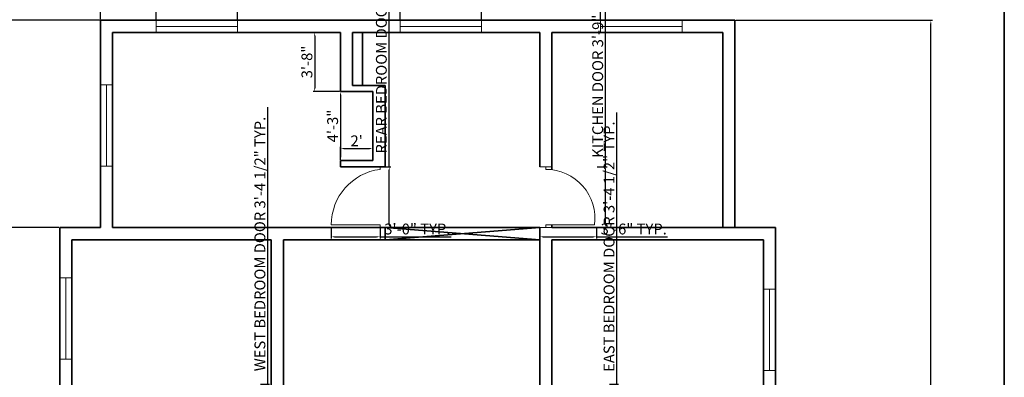
# Model space of a CAD drawing. Units: inches. Extents: x 2257 to 3678, y 834 to 1975.
# Tile 8 of 16: x 2952 to 3678, y 1330 to 1594. Entities that reach past the tile are written whole.
import ezdxf

# ---------------------------------------------------------------- set-up
doc = ezdxf.new("R2010")
doc.units = ezdxf.units.IN
for name, color, linetype, lineweight in [('A-ANNO-DIMS', 2, 'Continuous', 18), ('A-ANNO-TTLB', 7, 'Continuous', 35), ('A-DOOR', 3, 'Continuous', 18), ('A-GLAZ', 4, 'Continuous', 18), ('A-WALL', 7, 'Continuous', 35)]:
    doc.layers.add(name, color=color, linetype=linetype, lineweight=lineweight)
doc.styles.get("Standard").update_dxf_attribs({"font": 'arial.ttf'})
doc.dimstyles.new('ISO-25', dxfattribs={"dimtxt": 8, "dimasz": 2.5, "dimexe": 1.25, "dimexo": 0.625, "dimtad": 1, "dimdec": 0, "dimlunit": 3, "dimtxsty": 'Standard', "dimcen": 2.5, "dimadec": 0, "dimazin": 0, "dimtfac": 1, "dimtdec": 0, "dimtmove": 0, "dimatfit": 3, "dimfxl": 1, "dimarcsym": 0})

# ---------------------------------------------------------------- blocks, each defined once
blk = doc.blocks.new('*D17')
at = {"layer": 'A-ANNO-DIMS', "color": 0, "lineweight": -2, "transparency": 16777216}
for p, q in [((3187.62, 1584.58), (3168.03, 1584.58)), ((3169.28, 1582.08), (3169.28, 1543.58)), ((3187.62, 1541.08), (3168.03, 1541.08))]:
    blk.add_line(p, q, dxfattribs=at)
at = {"layer": 'A-ANNO-DIMS', "color": 0, "transparency": 16777216}
for points in [[(3168.87, 1582.08), (3169.7, 1582.08), (3169.28, 1584.58)], [(3168.87, 1543.58), (3169.7, 1543.58), (3169.28, 1541.08)]]:
    blk.add_solid(points, dxfattribs=at)
at = {"layer": 'Defpoints', "color": 0, "transparency": 16777216}
for p in [(3188.24, 1584.58), (3169.28, 1541.08), (3188.24, 1541.08)]:
    blk.add_point(p, dxfattribs=at)
at = {"layer": 'A-ANNO-DIMS', "color": 0, "transparency": 16777216, "insert": (3164.57, 1562.83), "char_height": 8, "attachment_point": 5, "rotation": 90}
blk.add_mtext('3\'-8"', dxfattribs=at)
blk = doc.blocks.new('*D18')
at = {"layer": 'A-ANNO-DIMS', "color": 0, "lineweight": -2, "transparency": 16777216}
for p, q in [((3188.87, 1541.08), (3189.49, 1541.08)), ((3188.24, 1538.58), (3188.24, 1492.58)), ((3188.87, 1490.08), (3189.49, 1490.08))]:
    blk.add_line(p, q, dxfattribs=at)
at = {"layer": 'A-ANNO-DIMS', "color": 0, "transparency": 16777216}
for points in [[(3187.82, 1538.58), (3188.66, 1538.58), (3188.24, 1541.08)], [(3187.82, 1492.58), (3188.66, 1492.58), (3188.24, 1490.08)]]:
    blk.add_solid(points, dxfattribs=at)
at = {"layer": 'Defpoints', "color": 0, "transparency": 16777216}
for p in [(3188.24, 1541.08), (3188.24, 1490.08), (3188.24, 1490.08)]:
    blk.add_point(p, dxfattribs=at)
at = {"layer": 'A-ANNO-DIMS', "color": 0, "transparency": 16777216, "insert": (3183.53, 1515.58), "char_height": 8, "attachment_point": 5, "rotation": 90}
blk.add_mtext('4\'-3"', dxfattribs=at)
blk = doc.blocks.new('*D15')
at = {"layer": 'A-ANNO-DIMS', "color": 0, "lineweight": -2, "transparency": 16777216}
for p, q in [((3188.24, 1490.7), (3188.24, 1500.22)), ((3190.74, 1498.97), (3209.74, 1498.97)), ((3212.24, 1490.7), (3212.24, 1500.22))]:
    blk.add_line(p, q, dxfattribs=at)
at = {"layer": 'A-ANNO-DIMS', "color": 0, "transparency": 16777216}
for points in [[(3190.74, 1499.38), (3190.74, 1498.55), (3188.24, 1498.97)], [(3209.74, 1499.38), (3209.74, 1498.55), (3212.24, 1498.97)]]:
    blk.add_solid(points, dxfattribs=at)
at = {"layer": 'Defpoints', "color": 0, "transparency": 16777216}
for p in [(3212.24, 1498.97), (3188.24, 1490.08), (3212.24, 1490.08)]:
    blk.add_point(p, dxfattribs=at)
at = {"layer": 'A-ANNO-DIMS', "color": 0, "transparency": 16777216, "insert": (3200.24, 1503.61), "char_height": 8, "attachment_point": 5}
blk.add_mtext("2'", dxfattribs=at)
blk = doc.blocks.new('WIN-60')
for p, q in [((0, 9), (0, 0)), ((60, 4.5), (60, 9)), ((60, 9), (60, 0)), ((0, 0), (0, 4.5)), ((0, 4.5), (60, 4.5))]:
    blk.add_line(p, q)
blk = doc.blocks.new('WIN-60-SIDE')
for p, q in [((0, 60), (9, 60)), ((9, 60), (4.5, 60)), ((4.5, 60), (4.5, 0)), ((9, 0), (0, 0)), ((4.5, 0), (9, 0))]:
    blk.add_line(p, q)
blk = doc.blocks.new('DOOR-BEDROOM-REAR')
for p, q in [((36, 45), (36, 43)), ((36, 2), (0, 2)), ((36, 0), (36, 2))]:
    blk.add_line(p, q)
blk.add_arc((41.35, 2), 41.35, 97.43058, 180)
blk = doc.blocks.new('DOOR-KITCHEN')
for p, q in [((0, 45), (9, 45)), ((4.5, 45), (4.5, 43)), ((9, 45), (4.5, 45)), ((4.5, 0), (4.5, 2)), ((4.5, 2), (40.5, 2)), ((9, 0), (0, 0))]:
    blk.add_line(p, q)
blk.add_arc((4.5, 6.7), 36.3, 352.56942, 90)
blk = doc.blocks.new('*D62')
at = {"layer": 'A-ANNO-DIMS', "color": 0, "lineweight": -2, "transparency": 16777216}
for p, q in [((3224.23, 1485.58), (3224.23, 1669.32)), ((3218.11, 1485.58), (3225.48, 1485.58)), ((3224.23, 1443.08), (3224.23, 1483.08)), ((3218.11, 1440.58), (3225.48, 1440.58))]:
    blk.add_line(p, q, dxfattribs=at)
at = {"layer": 'A-ANNO-DIMS', "color": 0, "transparency": 16777216}
for points in [[(3223.82, 1483.08), (3224.65, 1483.08), (3224.23, 1485.58)], [(3223.82, 1443.08), (3224.65, 1443.08), (3224.23, 1440.58)]]:
    blk.add_solid(points, dxfattribs=at)
at = {"layer": 'Defpoints', "color": 0, "transparency": 16777216}
for p in [(3217.48, 1485.58), (3224.23, 1485.58), (3217.48, 1440.58)]:
    blk.add_point(p, dxfattribs=at)
at = {"layer": 'A-ANNO-DIMS', "color": 0, "transparency": 16777216, "insert": (3219.47, 1578.7), "char_height": 8, "attachment_point": 5, "rotation": 90}
blk.add_mtext('REAR BEDROOM DOOR 3\'-9" TYP.', dxfattribs=at)
blk = doc.blocks.new('*D63')
at = {"layer": 'A-ANNO-DIMS', "color": 0, "lineweight": -2, "transparency": 16777216}
for p, q in [((3181.48, 1439.95), (3181.48, 1432.58)), ((3217.48, 1439.95), (3217.48, 1432.58)), ((3183.98, 1433.83), (3214.98, 1433.83)), ((3217.48, 1433.83), (3269.99, 1433.83))]:
    blk.add_line(p, q, dxfattribs=at)
at = {"layer": 'A-ANNO-DIMS', "color": 0, "transparency": 16777216}
for points in [[(3183.98, 1434.24), (3183.98, 1433.41), (3181.48, 1433.83)], [(3214.98, 1434.24), (3214.98, 1433.41), (3217.48, 1433.83)]]:
    blk.add_solid(points, dxfattribs=at)
at = {"layer": 'Defpoints', "color": 0, "transparency": 16777216}
for p in [(3181.48, 1440.58), (3217.48, 1440.58), (3217.48, 1433.83)]:
    blk.add_point(p, dxfattribs=at)
at = {"layer": 'A-ANNO-DIMS', "color": 0, "transparency": 16777216, "insert": (3244.99, 1438.54), "char_height": 8, "attachment_point": 5}
blk.add_mtext('3\'-0" TYP.', dxfattribs=at)
blk = doc.blocks.new('*D64')
at = {"layer": 'A-ANNO-DIMS', "color": 0, "lineweight": -2, "transparency": 16777216}
for p, q in [((3134.67, 1325.08), (3134.67, 1529.43)), ((3129.22, 1325.08), (3135.92, 1325.08)), ((3134.67, 1287.08), (3134.67, 1322.58)), ((3129.22, 1284.58), (3135.92, 1284.58))]:
    blk.add_line(p, q, dxfattribs=at)
at = {"layer": 'A-ANNO-DIMS', "color": 0, "transparency": 16777216}
for points in [[(3134.25, 1322.58), (3135.09, 1322.58), (3134.67, 1325.08)], [(3134.25, 1287.08), (3135.09, 1287.08), (3134.67, 1284.58)]]:
    blk.add_solid(points, dxfattribs=at)
at = {"layer": 'Defpoints', "color": 0, "transparency": 16777216}
for p in [(3128.6, 1325.08), (3134.67, 1325.08), (3128.6, 1284.58)]:
    blk.add_point(p, dxfattribs=at)
at = {"layer": 'A-ANNO-DIMS', "color": 0, "transparency": 16777216, "insert": (3129.9, 1428.5), "char_height": 8, "attachment_point": 5, "rotation": 90}
blk.add_mtext('WEST BEDROOM DOOR 3\'-4 1/2" TYP.', dxfattribs=at)
blk = doc.blocks.new('*D66')
at = {"layer": 'A-ANNO-DIMS', "color": 0, "lineweight": -2, "transparency": 16777216}
for p, q in [((3392.2, 1325.08), (3392.2, 1525.59)), ((3386.75, 1325.08), (3393.45, 1325.08)), ((3392.2, 1287.08), (3392.2, 1322.58)), ((3386.75, 1284.58), (3393.45, 1284.58))]:
    blk.add_line(p, q, dxfattribs=at)
at = {"layer": 'A-ANNO-DIMS', "color": 0, "transparency": 16777216}
for points in [[(3391.79, 1322.58), (3392.62, 1322.58), (3392.2, 1325.08)], [(3391.79, 1287.08), (3392.62, 1287.08), (3392.2, 1284.58)]]:
    blk.add_solid(points, dxfattribs=at)
at = {"layer": 'Defpoints', "color": 0, "transparency": 16777216}
for p in [(3386.13, 1325.08), (3392.2, 1325.08), (3386.13, 1284.58)]:
    blk.add_point(p, dxfattribs=at)
at = {"layer": 'A-ANNO-DIMS', "color": 0, "transparency": 16777216, "insert": (3387.44, 1426.58), "char_height": 8, "attachment_point": 5, "rotation": 90}
blk.add_mtext('EAST BEDROOM DOOR 3\'-4 1/2" TYP.', dxfattribs=at)
blk = doc.blocks.new('*D70')
at = {"layer": 'A-ANNO-DIMS', "color": 0, "lineweight": -2, "transparency": 16777216}
for p, q in [((3383.84, 1485.58), (3383.84, 1626.53)), ((3377.72, 1485.58), (3385.09, 1485.58)), ((3383.84, 1443.08), (3383.84, 1483.08)), ((3377.72, 1440.58), (3385.09, 1440.58))]:
    blk.add_line(p, q, dxfattribs=at)
at = {"layer": 'A-ANNO-DIMS', "color": 0, "transparency": 16777216}
for points in [[(3383.42, 1483.08), (3384.26, 1483.08), (3383.84, 1485.58)], [(3383.42, 1443.08), (3384.26, 1443.08), (3383.84, 1440.58)]]:
    blk.add_solid(points, dxfattribs=at)
at = {"layer": 'Defpoints', "color": 0, "transparency": 16777216}
for p in [(3377.09, 1485.58), (3383.84, 1485.58), (3377.09, 1440.58)]:
    blk.add_point(p, dxfattribs=at)
at = {"layer": 'A-ANNO-DIMS', "color": 0, "transparency": 16777216, "insert": (3379.07, 1557.3), "char_height": 8, "attachment_point": 5, "rotation": 90}
blk.add_mtext('KITCHEN DOOR 3\'-9" TYP.', dxfattribs=at)
blk = doc.blocks.new('*D71')
at = {"layer": 'A-ANNO-DIMS', "color": 0, "lineweight": -2, "transparency": 16777216}
for p, q in [((3335.24, 1439.95), (3335.24, 1432.58)), ((3377.09, 1439.95), (3377.09, 1432.58)), ((3337.74, 1433.83), (3374.59, 1433.83)), ((3377.09, 1433.83), (3429.6, 1433.83))]:
    blk.add_line(p, q, dxfattribs=at)
at = {"layer": 'A-ANNO-DIMS', "color": 0, "transparency": 16777216}
for points in [[(3337.74, 1434.24), (3337.74, 1433.41), (3335.24, 1433.83)], [(3374.59, 1434.24), (3374.59, 1433.41), (3377.09, 1433.83)]]:
    blk.add_solid(points, dxfattribs=at)
at = {"layer": 'Defpoints', "color": 0, "transparency": 16777216}
for p in [(3335.24, 1440.58), (3377.09, 1440.58), (3377.09, 1433.83)]:
    blk.add_point(p, dxfattribs=at)
at = {"layer": 'A-ANNO-DIMS', "color": 0, "transparency": 16777216, "insert": (3404.6, 1438.54), "char_height": 8, "attachment_point": 5}
blk.add_mtext('3\'-6" TYP.', dxfattribs=at)
blk = doc.blocks.new('*D100')
at = {"layer": 'A-ANNO-DIMS', "color": 0, "lineweight": -2, "transparency": 16777216}
for p, q in [((3479.87, 1593.58), (3625.01, 1593.58)), ((3623.76, 931.6), (3623.76, 1591.08)), ((3369.06, 929.1), (3625.01, 929.1))]:
    blk.add_line(p, q, dxfattribs=at)
at = {"layer": 'A-ANNO-DIMS', "color": 0, "transparency": 16777216}
for points in [[(3623.34, 1591.08), (3624.17, 1591.08), (3623.76, 1593.58)], [(3623.34, 931.6), (3624.17, 931.6), (3623.76, 929.1)]]:
    blk.add_solid(points, dxfattribs=at)
at = {"layer": 'Defpoints', "color": 0, "transparency": 16777216}
for p in [(3479.24, 1593.58), (3623.76, 1593.58), (3368.44, 929.1)]:
    blk.add_point(p, dxfattribs=at)
at = {"layer": 'A-ANNO-DIMS', "color": 0, "transparency": 16777216, "insert": (3618.99, 1261.34), "char_height": 8, "attachment_point": 5, "rotation": 90}
blk.add_mtext('55\'-4 1/2"', dxfattribs=at)
blk = doc.blocks.new('*D103')
at = {"layer": 'A-ANNO-DIMS', "color": 0, "lineweight": -2, "transparency": 16777216}
for p, q in [((2980.62, 1440.58), (2896.72, 1440.58)), ((2897.97, 1287.08), (2897.97, 1438.08)), ((2980.62, 1284.58), (2896.72, 1284.58))]:
    blk.add_line(p, q, dxfattribs=at)
at = {"layer": 'A-ANNO-DIMS', "color": 0, "transparency": 16777216}
for points in [[(2897.55, 1438.08), (2898.38, 1438.08), (2897.97, 1440.58)], [(2897.55, 1287.08), (2898.38, 1287.08), (2897.97, 1284.58)]]:
    blk.add_solid(points, dxfattribs=at)
at = {"layer": 'Defpoints', "color": 0, "transparency": 16777216}
for p in [(2897.97, 1440.58), (2981.24, 1440.58), (2981.24, 1284.58)]:
    blk.add_point(p, dxfattribs=at)
at = {"layer": 'A-ANNO-DIMS', "color": 0, "transparency": 16777216, "insert": (2893.25, 1362.58), "char_height": 8, "attachment_point": 5, "rotation": 90}
blk.add_mtext('13\'-0"', dxfattribs=at)
blk = doc.blocks.new('*D104')
at = {"layer": 'A-ANNO-DIMS', "color": 0, "lineweight": -2, "transparency": 16777216}
for p, q in [((3010.62, 1593.58), (2896.72, 1593.58)), ((2897.97, 1443.08), (2897.97, 1591.08)), ((2980.62, 1440.58), (2896.72, 1440.58))]:
    blk.add_line(p, q, dxfattribs=at)
at = {"layer": 'A-ANNO-DIMS', "color": 0, "transparency": 16777216}
for points in [[(2897.55, 1591.08), (2898.38, 1591.08), (2897.97, 1593.58)], [(2897.55, 1443.08), (2898.38, 1443.08), (2897.97, 1440.58)]]:
    blk.add_solid(points, dxfattribs=at)
at = {"layer": 'Defpoints', "color": 0, "transparency": 16777216}
for p in [(2897.97, 1593.58), (3011.24, 1593.58), (2981.24, 1440.58)]:
    blk.add_point(p, dxfattribs=at)
at = {"layer": 'A-ANNO-DIMS', "color": 0, "transparency": 16777216, "insert": (2893.26, 1517.08), "char_height": 8, "attachment_point": 5, "rotation": 90}
blk.add_mtext('12\'-9"', dxfattribs=at)
blk = doc.blocks.new('*D108')
at = {"layer": 'A-ANNO-DIMS', "color": 0, "lineweight": -2, "transparency": 16777216}
for p, q in [((3011.24, 1594.2), (3011.24, 1628.38)), ((3013.74, 1627.13), (3049.79, 1627.13)), ((3052.29, 1594.2), (3052.29, 1628.38))]:
    blk.add_line(p, q, dxfattribs=at)
at = {"layer": 'A-ANNO-DIMS', "color": 0, "transparency": 16777216}
for points in [[(3013.74, 1627.54), (3013.74, 1626.71), (3011.24, 1627.13)], [(3049.79, 1627.54), (3049.79, 1626.71), (3052.29, 1627.13)]]:
    blk.add_solid(points, dxfattribs=at)
at = {"layer": 'Defpoints', "color": 0, "transparency": 16777216}
for p in [(3052.29, 1627.13), (3011.24, 1593.58), (3052.29, 1593.58)]:
    blk.add_point(p, dxfattribs=at)
at = {"layer": 'A-ANNO-DIMS', "color": 0, "transparency": 16777216, "insert": (3031.77, 1631.84), "char_height": 8, "attachment_point": 5}
blk.add_mtext('3\'-5"', dxfattribs=at)
blk = doc.blocks.new('*D109')
at = {"layer": 'A-ANNO-DIMS', "color": 0, "lineweight": -2, "transparency": 16777216}
for p, q in [((3112.29, 1594.2), (3112.29, 1628.38)), ((3114.79, 1627.13), (3229.89, 1627.13)), ((3232.39, 1594.2), (3232.39, 1628.38))]:
    blk.add_line(p, q, dxfattribs=at)
at = {"layer": 'A-ANNO-DIMS', "color": 0, "transparency": 16777216}
for points in [[(3114.79, 1627.54), (3114.79, 1626.71), (3112.29, 1627.13)], [(3229.89, 1627.54), (3229.89, 1626.71), (3232.39, 1627.13)]]:
    blk.add_solid(points, dxfattribs=at)
at = {"layer": 'Defpoints', "color": 0, "transparency": 16777216}
for p in [(3232.39, 1627.13), (3112.29, 1593.58), (3232.39, 1593.58)]:
    blk.add_point(p, dxfattribs=at)
at = {"layer": 'A-ANNO-DIMS', "color": 0, "transparency": 16777216, "insert": (3172.34, 1631.84), "char_height": 8, "attachment_point": 5}
blk.add_mtext('10\'-0"', dxfattribs=at)
blk = doc.blocks.new('*D110')
at = {"layer": 'A-ANNO-DIMS', "color": 0, "lineweight": -2, "transparency": 16777216}
for p, q in [((3292.39, 1594.2), (3292.39, 1628.38)), ((3294.89, 1627.13), (3377.71, 1627.13)), ((3380.21, 1594.2), (3380.21, 1628.38))]:
    blk.add_line(p, q, dxfattribs=at)
at = {"layer": 'A-ANNO-DIMS', "color": 0, "transparency": 16777216}
for points in [[(3294.89, 1627.54), (3294.89, 1626.71), (3292.39, 1627.13)], [(3377.71, 1627.54), (3377.71, 1626.71), (3380.21, 1627.13)]]:
    blk.add_solid(points, dxfattribs=at)
at = {"layer": 'Defpoints', "color": 0, "transparency": 16777216}
for p in [(3380.21, 1627.13), (3292.39, 1593.58), (3380.21, 1593.58)]:
    blk.add_point(p, dxfattribs=at)
at = {"layer": 'A-ANNO-DIMS', "color": 0, "transparency": 16777216, "insert": (3336.3, 1631.75), "char_height": 8, "attachment_point": 5}
blk.add_mtext('7\'-4"', dxfattribs=at)

msp = doc.modelspace()

# ---------------------------------------------------------------- linework, layer by layer
at = {"layer": 'A-ANNO-TTLB'}
msp.add_lwpolyline([(2257.38, 1974.9), (3677.96, 1974.9), (3677.96, 849.42), (2257.38, 849.42)], close=True, dxfattribs=at)
at = {"layer": 'A-GLAZ'}
msp.add_line((2981.24, 1403.59), (2981.24, 1403.59), dxfattribs=at)
at = {"layer": 'A-WALL'}
for p, q in [((3011.24, 1593.58), (3011.24, 1440.58)), ((3011.24, 1593.58), (3479.24, 1593.58)), ((3011.24, 1593.58), (3292.39, 1593.58)), ((3335.24, 1593.58), (3479.24, 1593.58)), ((3479.24, 1593.58), (3479.24, 1440.58)), ((3020.24, 1584.58), (3020.24, 1440.58)), ((3020.24, 1584.58), (3188.24, 1584.58)), ((3188.24, 1584.58), (3188.24, 1541.08)), ((3197.24, 1584.58), (3197.24, 1545.58)), ((3197.24, 1584.58), (3335.24, 1584.58)), ((3197.24, 1584.58), (3197.24, 1545.58)), ((3204.55, 1545.58), (3204.55, 1584.58)), ((3335.24, 1584.58), (3335.24, 1485.58)), ((3344.24, 1584.58), (3344.24, 1483.3)), ((3344.24, 1584.58), (3470.24, 1584.58)), ((3470.24, 1584.58), (3470.24, 1440.58)), ((3212.24, 1541.08), (3188.24, 1541.08)), ((3197.24, 1545.58), (3221.24, 1545.58)), ((3212.24, 1490.08), (3212.24, 1541.08)), ((3221.24, 1545.58), (3221.24, 1485.58)), ((3188.24, 1490.08), (3188.24, 1485.58)), ((3188.24, 1485.58), (3188.24, 1490.08)), ((3188.24, 1490.08), (3212.24, 1490.08)), ((3221.24, 1485.58), (3188.24, 1485.58)), ((2981.24, 1440.58), (2981.24, 1284.58)), ((2981.24, 1440.58), (3011.24, 1440.58)), ((3020.24, 1440.58), (3335.24, 1440.58)), ((3221.24, 1440.58), (3221.24, 1431.58)), ((3221.24, 1440.58), (3335.24, 1431.58)), ((3335.24, 1440.58), (3221.24, 1431.58)), ((3335.24, 1440.58), (3335.24, 1431.58)), ((3335.24, 1431.58), (3335.24, 1440.58)), ((3335.24, 1440.58), (3335.24, 1440.58)), ((3344.24, 1442.58), (3344.24, 1440.58)), ((3344.24, 1440.58), (3470.24, 1440.58)), ((3470.24, 1440.58), (3509.24, 1440.58)), ((3509.24, 1440.58), (3509.24, 1431.58)), ((2990.24, 1431.58), (2990.24, 1293.58)), ((2990.24, 1431.58), (3137.24, 1431.58)), ((3137.24, 1431.58), (3137.24, 1293.58)), ((3146.24, 1431.58), (3146.24, 1172.08)), ((3146.24, 1431.58), (3335.24, 1431.58)), ((3335.24, 1431.58), (3335.24, 1172.08)), ((3335.24, 1431.58), (3335.24, 1172.08)), ((3344.24, 1431.58), (3344.24, 1172.08)), ((3344.24, 1431.58), (3470.24, 1431.58)), ((3470.24, 1431.58), (3500.24, 1431.58)), ((3500.24, 1431.58), (3500.24, 1293.58)), ((3509.24, 1431.58), (3509.24, 1284.58))]:
    msp.add_line(p, q, dxfattribs=at)

# ---------------------------------------------------------------- block references
at = {"layer": 'A-DOOR'}
for name, p in [('DOOR-BEDROOM-REAR', (3181.48, 1440.58)), ('DOOR-KITCHEN', (3335.24, 1440.58))]:
    msp.add_blockref(name, p, dxfattribs=at)
at = {"layer": 'A-GLAZ'}
for name, p in [('WIN-60', (3052.29, 1584.58)), ('WIN-60', (3232.39, 1584.58)), ('WIN-60', (3380.21, 1584.58)), ('WIN-60-SIDE', (3011.24, 1485.89))]:
    msp.add_blockref(name, p, dxfattribs=at)
at = {"layer": 'A-GLAZ', "extrusion": (0, 0, -1), "zscale": -1}
for p, rotation in [((-2990.24, 1403.59), 270.0000000000027), ((-3509.24, 1395.2), 270.0000000000025)]:
    msp.add_blockref('WIN-60', p, dxfattribs=dict(at, rotation=rotation))

# ---------------------------------------------------------------- dimensions: what is measured, and where the dimension line sits
at = {"layer": 'A-ANNO-DIMS'}
for base, p1, p2, text, picture, middle in [((3224.23, 1485.58), (3217.48, 1440.58), (3217.48, 1485.58), 'REAR BEDROOM DOOR <> TYP.', '*D62', (3219.47, 1578.7)), ((3383.84, 1485.58), (3377.09, 1440.58), (3377.09, 1485.58), 'KITCHEN DOOR <> TYP.', '*D70', (3379.07, 1557.3)), ((3134.67, 1325.08), (3128.6, 1284.58), (3128.6, 1325.08), 'WEST BEDROOM DOOR <> TYP.', '*D64', (3129.9, 1428.5)), ((3392.2, 1325.08), (3386.13, 1284.58), (3386.13, 1325.08), 'EAST BEDROOM DOOR <> TYP.', '*D66', (3387.44, 1426.58))]:
    dim = msp.add_linear_dim(base=base, p1=p1, p2=p2, angle=90, text=text, dimstyle='ISO-25', override={"dimdec": 1, "dimlfac": 1, "dimrnd": 0, "dimzin": 1, "dimdsep": 46, "dimlunit": 4, "dimfrac": 2}, dxfattribs=at)
    dim.commit()
    dim.dimension.update_dxf_attribs({"geometry": picture, "text_midpoint": middle})
for base, p1, p2, override, picture, middle in [((3052.2934, 1627.1269), (3011.2405, 1593.5769), (3052.2934, 1593.5769), {"dimdec": 1, "dimlfac": 1, "dimrnd": 0, "dimzin": 1, "dimdsep": 46, "dimlunit": 4, "dimfrac": 2}, '*D108', (3031.7669, 1631.8393)), ((3232.39, 1627.13), (3112.29, 1593.58), (3232.39, 1593.58), {"dimdec": 1, "dimlfac": 1, "dimrnd": 0, "dimzin": 1, "dimdsep": 46, "dimlunit": 4, "dimfrac": 2}, '*D109', (3172.34, 1631.84)), ((3380.21, 1627.13), (3292.39, 1593.58), (3380.21, 1593.58), {"dimdec": 1, "dimlfac": 1, "dimrnd": 0, "dimzin": 1, "dimdsep": 46, "dimlunit": 4, "dimfrac": 2}, '*D110', (3336.3, 1631.75)), ((3212.24, 1498.97), (3188.24, 1490.08), (3212.24, 1490.08), {"dimclrd": 0, "dimclre": 0, "dimclrt": 0}, '*D15', (3200.24, 1503.61))]:
    dim = msp.add_linear_dim(base=base, p1=p1, p2=p2, dimstyle='ISO-25', override=override, dxfattribs=at)
    dim.commit()
    dim.dimension.update_dxf_attribs({"geometry": picture, "text_midpoint": middle})
for base, p1, p2, override, picture, middle in [((2897.97, 1593.58), (2981.24, 1440.58), (3011.24, 1593.58), {"dimdec": 1, "dimlfac": 1, "dimrnd": 0, "dimzin": 1, "dimdsep": 46, "dimlunit": 4, "dimfrac": 2}, '*D104', (2893.26, 1517.08)), ((3623.76, 1593.58), (3368.44, 929.1), (3479.24, 1593.58), {"dimdec": 1, "dimlfac": 1, "dimrnd": 0, "dimzin": 1, "dimdsep": 46, "dimlunit": 4, "dimfrac": 2}, '*D100', (3618.99, 1261.34)), ((3169.28280464, 1541.07694214), (3188.24045238, 1584.57694214), (3188.24045238, 1541.07694214), {"dimclrd": 0, "dimclre": 0, "dimclrt": 0}, '*D17', (3164.57049222, 1562.82694214)), ((3188.24, 1490.08), (3188.24, 1541.08), (3188.24, 1490.08), {"dimclrd": 0, "dimclre": 0, "dimclrt": 0}, '*D18', (3183.53, 1515.58)), ((2897.97, 1440.58), (2981.24, 1284.58), (2981.24, 1440.58), {"dimdec": 1, "dimlfac": 1, "dimrnd": 0, "dimzin": 1, "dimdsep": 46, "dimlunit": 4, "dimfrac": 2}, '*D103', (2893.25, 1362.58))]:
    dim = msp.add_linear_dim(base=base, p1=p1, p2=p2, angle=90, dimstyle='ISO-25', override=override, dxfattribs=at)
    dim.commit()
    dim.dimension.update_dxf_attribs({"geometry": picture, "text_midpoint": middle})
for base, p1, p2, picture, middle in [((3217.48, 1433.83), (3181.48, 1440.58), (3217.48, 1440.58), '*D63', (3244.99, 1438.54)), ((3377.0915, 1433.8269), (3335.2405, 1440.5769), (3377.0915, 1440.5769), '*D71', (3404.5958, 1438.5393))]:
    dim = msp.add_linear_dim(base=base, p1=p1, p2=p2, text='<> TYP.', dimstyle='ISO-25', override={"dimdec": 1, "dimlfac": 1, "dimrnd": 0, "dimzin": 1, "dimdsep": 46, "dimlunit": 4, "dimfrac": 2}, dxfattribs=at)
    dim.commit()
    dim.dimension.update_dxf_attribs({"geometry": picture, "text_midpoint": middle})

doc.saveas('drawing.dxf')
